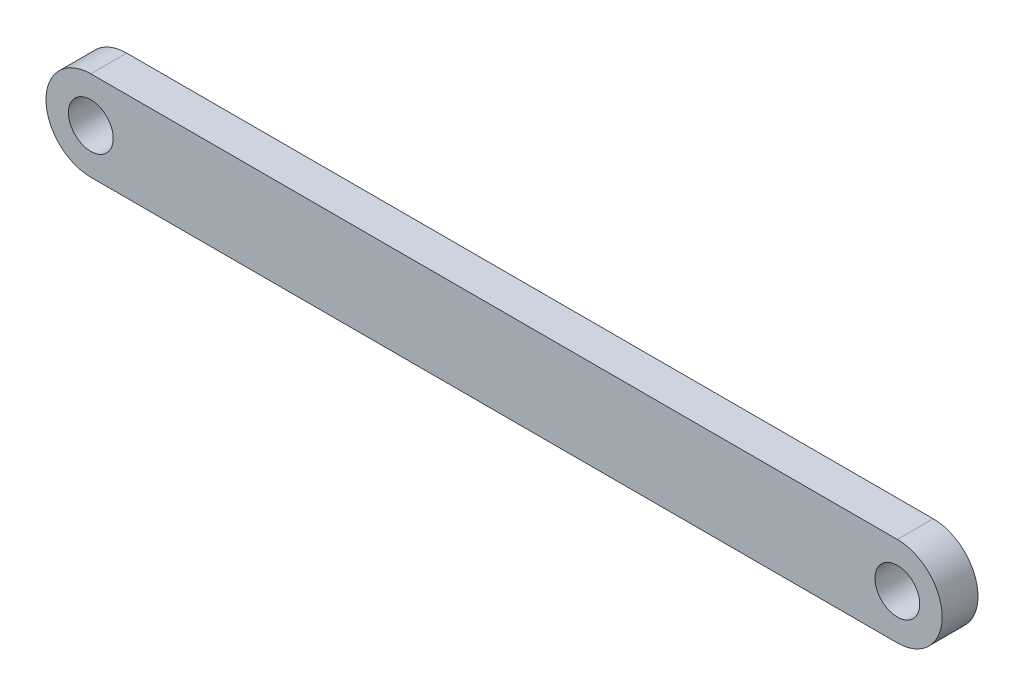
from build123d import *

# Parameters (mm, degrees)
LINK_PROFILE_SKETCH_R = 2.5
LINK_BAR_4MM_DEPTH    = 2


with BuildPart() as part:
    # Link Profile Sketch → Link Bar 4mm (new, symmetric)
    with BuildSketch(Plane.XY):
        with BuildLine():
            Line((-45, 5), (45, 5))
            ThreePointArc((45, 5), (50, 0), (45, -5))
            Line((45, -5), (-45, -5))
            ThreePointArc((-45, -5), (-50, 0), (-45, 5))
        make_face()
        with Locations((-45, 0)):
            Circle(LINK_PROFILE_SKETCH_R, mode=Mode.SUBTRACT)
        with Locations((45, 0)):
            Circle(LINK_PROFILE_SKETCH_R, mode=Mode.SUBTRACT)
    extrude(amount=LINK_BAR_4MM_DEPTH, both=True)


solid = part.part
